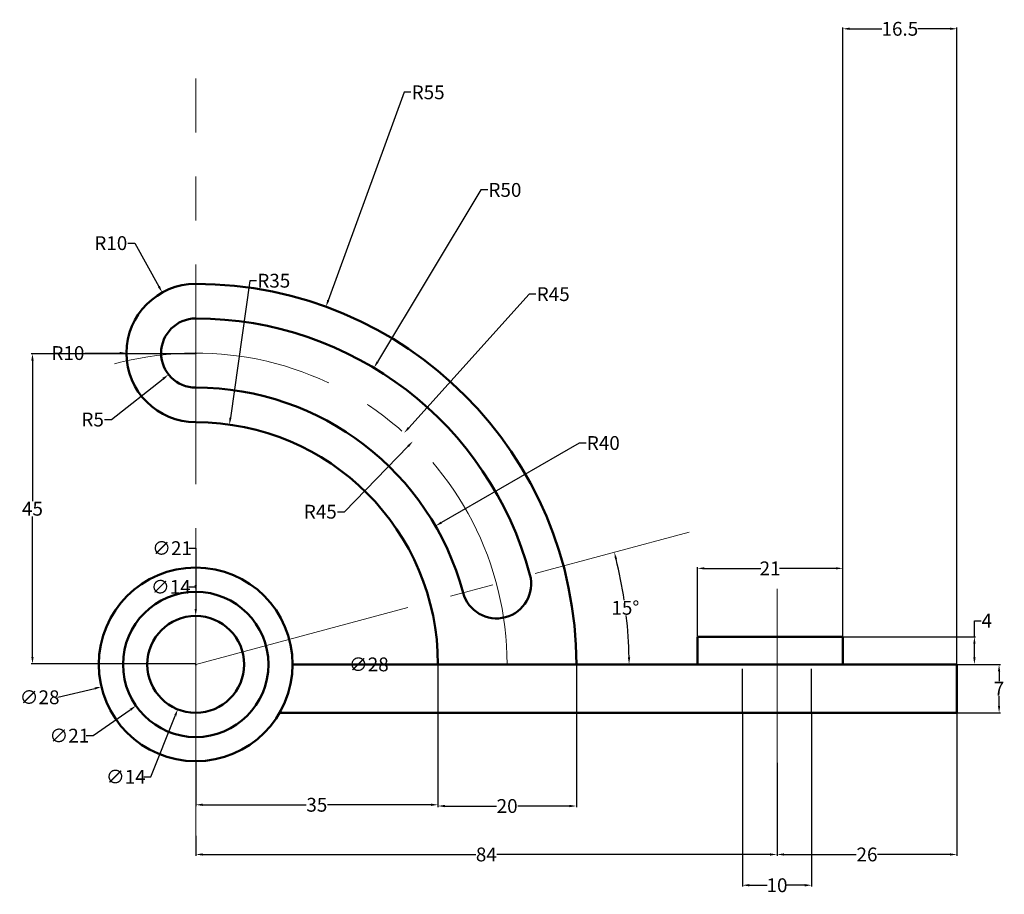
# Model space of a CAD drawing. Units: inches. Extents: x 69 to 212, y 27 to 154.
import ezdxf

# ---------------------------------------------------------------- set-up
doc = ezdxf.new("R2010")
doc.units = ezdxf.units.IN
doc.header["$MEASUREMENT"] = 0
doc.linetypes.add('CENTER', pattern=[50.8, 31.75, -6.35, 6.35, -6.35])
doc.linetypes.add('HIDDEN', pattern=[9.525, 6.35, -3.175])
for name, color, linetype, lineweight in [('M-CNTR', 4, 'CENTER', 18), ('M-DIMS', 2, 'Continuous', 25), ('M-HIDN', 3, 'HIDDEN', 25), ('M-OUTL', 7, 'Continuous', 50)]:
    doc.layers.add(name, color=color, linetype=linetype, lineweight=lineweight)
doc.styles.get("Standard").update_dxf_attribs({"font": 'arial.ttf'})
doc.dimstyles.get("Standard").update_dxf_attribs({"dimtxt": 2, "dimasz": 1, "dimexe": 0.18, "dimexo": 0.0625, "dimgap": 0.09, "dimtad": 0, "dimtih": 1, "dimtoh": 1, "dimdec": 0, "dimzin": 0, "dimdsep": 46, "dimtxsty": 'Standard', "dimcen": 0.09, "dimclrd": 1, "dimclre": 1, "dimadec": 0, "dimazin": 0, "dimtfac": 1, "dimtdec": 0, "dimtofl": 0, "dimtmove": 0, "dimatfit": 3, "dimfxl": 1, "dimtolj": 1, "dimtzin": 0, "dimarcsym": 0})

# ---------------------------------------------------------------- blocks, each defined once
blk = doc.blocks.new('*D1')
at = {"layer": 'Defpoints', "color": 0, "transparency": 16777216}
for p in [(108.33, 63.95), (81.09, 57.47)]:
    blk.add_point(p, dxfattribs=at)
at = {"layer": 'M-DIMS', "color": 0, "lineweight": -2, "transparency": 16777216}
for p, q in [((94.62, 60.71), (94.8, 60.71)), ((94.71, 60.62), (94.71, 60.8)), ((74.77, 55.96), (80.12, 57.24))]:
    blk.add_line(p, q, dxfattribs=at)
at = {"layer": 'M-DIMS', "color": 0, "transparency": 16777216}
blk.add_solid([(80.08, 57.4), (80.16, 57.08), (81.09, 57.47)], dxfattribs=at)
at = {"layer": 'M-DIMS', "color": 0, "transparency": 16777216, "insert": (72.15, 55.96), "char_height": 2, "attachment_point": 5}
blk.add_mtext('\\A1;∅28', dxfattribs=at)
blk = doc.blocks.new('*D2')
at = {"layer": 'Defpoints', "color": 0, "transparency": 16777216}
for p in [(103.34, 66.7), (86.08, 54.73)]:
    blk.add_point(p, dxfattribs=at)
at = {"layer": 'M-DIMS', "color": 0, "lineweight": -2, "transparency": 16777216}
for p, q in [((94.62, 60.71), (94.8, 60.71)), ((94.71, 60.62), (94.71, 60.8)), ((79.87, 50.41), (85.26, 54.16)), ((78.87, 50.41), (79.87, 50.41))]:
    blk.add_line(p, q, dxfattribs=at)
at = {"layer": 'M-DIMS', "color": 0, "transparency": 16777216}
blk.add_solid([(85.17, 54.29), (85.36, 54.02), (86.08, 54.73)], dxfattribs=at)
at = {"layer": 'M-DIMS', "color": 0, "transparency": 16777216, "insert": (76.45, 50.41), "char_height": 2, "attachment_point": 5}
blk.add_mtext('\\A1;∅21', dxfattribs=at)
blk = doc.blocks.new('*D3')
at = {"layer": 'Defpoints', "color": 0, "transparency": 16777216}
for p in [(97.31, 67.21), (92.11, 54.21)]:
    blk.add_point(p, dxfattribs=at)
at = {"layer": 'M-DIMS', "color": 0, "lineweight": -2, "transparency": 16777216}
for p, q in [((94.62, 60.71), (94.8, 60.71)), ((94.71, 60.62), (94.71, 60.8)), ((88.21, 44.47), (91.74, 53.28)), ((87.21, 44.47), (88.21, 44.47))]:
    blk.add_line(p, q, dxfattribs=at)
at = {"layer": 'M-DIMS', "color": 0, "transparency": 16777216}
blk.add_solid([(91.59, 53.35), (91.9, 53.22), (92.11, 54.21)], dxfattribs=at)
at = {"layer": 'M-DIMS', "color": 0, "transparency": 16777216, "insert": (84.61, 44.47), "char_height": 2, "attachment_point": 5}
blk.add_mtext('\\A1;∅14', dxfattribs=at)
blk = doc.blocks.new('*D4')
at = {"layer": 'Defpoints', "color": 0, "transparency": 16777216}
for p in [(129.71, 60.71), (94.71, 46.71), (94.71, 40.42)]:
    blk.add_point(p, dxfattribs=at)
at = {"layer": 'M-DIMS', "color": 0, "lineweight": -2, "transparency": 16777216}
for p, q in [((129.71, 60.65), (129.71, 40.24)), ((94.71, 46.65), (94.71, 40.24)), ((95.71, 40.42), (110.68, 40.42)), ((128.71, 40.42), (113.74, 40.42))]:
    blk.add_line(p, q, dxfattribs=at)
at = {"layer": 'M-DIMS', "color": 0, "transparency": 16777216}
for points in [[(95.71, 40.59), (95.71, 40.25), (94.71, 40.42)], [(128.71, 40.59), (128.71, 40.25), (129.71, 40.42)]]:
    blk.add_solid(points, dxfattribs=at)
at = {"layer": 'M-DIMS', "color": 0, "transparency": 16777216, "insert": (112.21, 40.42), "char_height": 2, "attachment_point": 5}
blk.add_mtext('\\A1;35', dxfattribs=at)
blk = doc.blocks.new('*D5')
at = {"layer": 'Defpoints', "color": 0, "transparency": 16777216}
for p in [(129.71, 60.71), (149.71, 60.71), (129.71, 40.24)]:
    blk.add_point(p, dxfattribs=at)
at = {"layer": 'M-DIMS', "color": 0, "lineweight": -2, "transparency": 16777216}
for p, q in [((129.71, 60.65), (129.71, 40.06)), ((149.71, 60.65), (149.71, 40.06)), ((130.71, 40.24), (138.18, 40.24)), ((148.71, 40.24), (141.25, 40.24))]:
    blk.add_line(p, q, dxfattribs=at)
at = {"layer": 'M-DIMS', "color": 0, "transparency": 16777216}
for points in [[(130.71, 40.41), (130.71, 40.07), (129.71, 40.24)], [(148.71, 40.41), (148.71, 40.07), (149.71, 40.24)]]:
    blk.add_solid(points, dxfattribs=at)
at = {"layer": 'M-DIMS', "color": 0, "transparency": 16777216, "insert": (139.71, 40.24), "char_height": 2, "attachment_point": 5}
blk.add_mtext('\\A1;20', dxfattribs=at)
blk = doc.blocks.new('*D6')
at = {"layer": 'Defpoints', "color": 0, "transparency": 16777216}
for p in [(178.71, 46.52), (94.71, 35.97), (178.71, 33.24)]:
    blk.add_point(p, dxfattribs=at)
at = {"layer": 'M-DIMS', "color": 0, "lineweight": -2, "transparency": 16777216}
for p, q in [((178.71, 46.46), (178.71, 33.06)), ((94.71, 35.91), (94.71, 33.06)), ((95.71, 33.24), (135.19, 33.24)), ((177.71, 33.24), (138.23, 33.24))]:
    blk.add_line(p, q, dxfattribs=at)
at = {"layer": 'M-DIMS', "color": 0, "transparency": 16777216}
for points in [[(95.71, 33.4), (95.71, 33.07), (94.71, 33.24)], [(177.71, 33.4), (177.71, 33.07), (178.71, 33.24)]]:
    blk.add_solid(points, dxfattribs=at)
at = {"layer": 'M-DIMS', "color": 0, "transparency": 16777216, "insert": (136.71, 33.24), "char_height": 2, "attachment_point": 5}
blk.add_mtext('\\A1;84', dxfattribs=at)
blk = doc.blocks.new('*D7')
at = {"layer": 'Defpoints', "color": 0, "transparency": 16777216}
for p in [(204.71, 53.71), (178.71, 46.52), (204.71, 33.24)]:
    blk.add_point(p, dxfattribs=at)
at = {"layer": 'M-DIMS', "color": 0, "lineweight": -2, "transparency": 16777216}
for p, q in [((204.71, 53.65), (204.71, 33.06)), ((178.71, 46.46), (178.71, 33.06)), ((179.71, 33.24), (190.17, 33.24)), ((203.71, 33.24), (193.25, 33.24))]:
    blk.add_line(p, q, dxfattribs=at)
at = {"layer": 'M-DIMS', "color": 0, "transparency": 16777216}
for points in [[(179.71, 33.4), (179.71, 33.07), (178.71, 33.24)], [(203.71, 33.4), (203.71, 33.07), (204.71, 33.24)]]:
    blk.add_solid(points, dxfattribs=at)
at = {"layer": 'M-DIMS', "color": 0, "transparency": 16777216, "insert": (191.71, 33.24), "char_height": 2, "attachment_point": 5}
blk.add_mtext('\\A1;26', dxfattribs=at)
blk = doc.blocks.new('*D8')
at = {"layer": 'Defpoints', "color": 0, "transparency": 16777216}
for p in [(204.71, 60.71), (204.71, 53.71), (210.8, 53.71)]:
    blk.add_point(p, dxfattribs=at)
at = {"layer": 'M-DIMS', "color": 0, "lineweight": -2, "transparency": 16777216}
for p, q in [((204.77, 60.71), (210.98, 60.71)), ((210.8, 59.71), (210.8, 58.3)), ((210.8, 54.71), (210.8, 56.12)), ((204.77, 53.71), (210.98, 53.71))]:
    blk.add_line(p, q, dxfattribs=at)
at = {"layer": 'M-DIMS', "color": 0, "transparency": 16777216}
for points in [[(210.63, 59.71), (210.96, 59.71), (210.8, 60.71)], [(210.63, 54.71), (210.96, 54.71), (210.8, 53.71)]]:
    blk.add_solid(points, dxfattribs=at)
at = {"layer": 'M-DIMS', "color": 0, "transparency": 16777216, "insert": (210.8, 57.21), "char_height": 2, "attachment_point": 5}
blk.add_mtext('\\A1;7', dxfattribs=at)
blk = doc.blocks.new('*D9')
at = {"layer": 'Defpoints', "color": 0, "transparency": 16777216}
for p in [(188.21, 64.71), (188.21, 60.71), (207.23, 60.71)]:
    blk.add_point(p, dxfattribs=at)
at = {"layer": 'M-DIMS', "color": 0, "lineweight": -2, "transparency": 16777216}
for p, q in [((207.23, 64.71), (207.23, 67.02)), ((207.23, 67.02), (208.23, 67.02)), ((188.27, 64.71), (207.41, 64.71)), ((207.23, 61.71), (207.23, 63.71)), ((188.27, 60.71), (207.41, 60.71))]:
    blk.add_line(p, q, dxfattribs=at)
at = {"layer": 'M-DIMS', "color": 0, "transparency": 16777216}
for points in [[(207.07, 63.71), (207.4, 63.71), (207.23, 64.71)], [(207.07, 61.71), (207.4, 61.71), (207.23, 60.71)]]:
    blk.add_solid(points, dxfattribs=at)
at = {"layer": 'M-DIMS', "color": 0, "transparency": 16777216, "insert": (209.01, 67.02), "char_height": 2, "attachment_point": 5}
blk.add_mtext('\\A1;4', dxfattribs=at)
blk = doc.blocks.new('*D10')
at = {"layer": 'Defpoints', "color": 0, "transparency": 16777216}
for p in [(188.21, 74.59), (167.21, 64.71), (188.21, 64.71)]:
    blk.add_point(p, dxfattribs=at)
at = {"layer": 'M-DIMS', "color": 0, "lineweight": -2, "transparency": 16777216}
for p, q in [((167.21, 64.77), (167.21, 74.77)), ((168.21, 74.59), (176.37, 74.59)), ((187.21, 74.59), (179.06, 74.59)), ((188.21, 64.77), (188.21, 74.77))]:
    blk.add_line(p, q, dxfattribs=at)
at = {"layer": 'M-DIMS', "color": 0, "transparency": 16777216}
for points in [[(168.21, 74.76), (168.21, 74.43), (167.21, 74.59)], [(187.21, 74.76), (187.21, 74.43), (188.21, 74.59)]]:
    blk.add_solid(points, dxfattribs=at)
at = {"layer": 'M-DIMS', "color": 0, "transparency": 16777216, "insert": (177.71, 74.59), "char_height": 2, "attachment_point": 5}
blk.add_mtext('\\A1;21', dxfattribs=at)
blk = doc.blocks.new('*D11')
at = {"layer": 'Defpoints', "color": 0, "transparency": 16777216}
for p in [(166.01, 79.82), (157.1, 66.17), (94.71, 60.71), (108.71, 60.71), (178.71, 60.71)]:
    blk.add_point(p, dxfattribs=at)
at = {"layer": 'M-DIMS', "color": 0, "lineweight": -2, "transparency": 16777216}
for start, end in [(8.5267, 14.085), (0.915, 6.4757)]:
    blk.add_arc((94.71, 60.71), 62.62, start, end, dxfattribs=at)
at = {"layer": 'M-DIMS', "color": 0, "transparency": 16777216}
for points in [[(155.29, 75.91), (155.61, 75.99), (155.2, 76.92)], [(157.49, 61.71), (157.16, 61.71), (157.33, 60.71)]]:
    blk.add_solid(points, dxfattribs=at)
at = {"layer": 'M-DIMS', "color": 0, "transparency": 16777216, "insert": (156.8, 68.89), "char_height": 2, "attachment_point": 5}
blk.add_mtext('\\A1;15°', dxfattribs=at)
blk = doc.blocks.new('*D12')
at = {"layer": 'Defpoints', "color": 0, "transparency": 16777216}
for p in [(126.1, 92.96), (94.71, 60.71)]:
    blk.add_point(p, dxfattribs=at)
at = {"layer": 'M-DIMS', "color": 0, "lineweight": -2, "transparency": 16777216}
for p, q in [((116.19, 82.78), (125.4, 92.24)), ((115.19, 82.78), (116.19, 82.78))]:
    blk.add_line(p, q, dxfattribs=at)
at = {"layer": 'M-DIMS', "color": 0, "transparency": 16777216}
blk.add_solid([(125.28, 92.36), (125.52, 92.12), (126.1, 92.96)], dxfattribs=at)
at = {"layer": 'M-DIMS', "color": 0, "transparency": 16777216, "insert": (112.71, 82.78), "char_height": 2, "attachment_point": 5}
blk.add_mtext('\\A1;R45', dxfattribs=at)
blk = doc.blocks.new('*D13')
at = {"layer": 'Defpoints', "color": 0, "transparency": 16777216}
for p in [(94.71, 105.71), (90.79, 102.61)]:
    blk.add_point(p, dxfattribs=at)
at = {"layer": 'M-DIMS', "color": 0, "lineweight": -2, "transparency": 16777216}
for p, q in [((94.62, 105.71), (94.8, 105.71)), ((94.71, 105.62), (94.71, 105.8)), ((82.53, 96.1), (90, 101.99)), ((81.53, 96.1), (82.53, 96.1))]:
    blk.add_line(p, q, dxfattribs=at)
at = {"layer": 'M-DIMS', "color": 0, "transparency": 16777216}
blk.add_solid([(89.9, 102.13), (90.11, 101.86), (90.79, 102.61)], dxfattribs=at)
at = {"layer": 'M-DIMS', "color": 0, "transparency": 16777216, "insert": (79.82, 96.1), "char_height": 2, "attachment_point": 5}
blk.add_mtext('\\A1;R5', dxfattribs=at)
blk = doc.blocks.new('*D14')
at = {"layer": 'Defpoints', "color": 0, "transparency": 16777216}
for p in [(89.87, 114.46), (94.71, 105.71)]:
    blk.add_point(p, dxfattribs=at)
at = {"layer": 'M-DIMS', "color": 0, "lineweight": -2, "transparency": 16777216}
for p, q in [((84.91, 121.6), (85.91, 121.6)), ((85.91, 121.6), (89.38, 115.34)), ((94.62, 105.71), (94.8, 105.71)), ((94.71, 105.62), (94.71, 105.8))]:
    blk.add_line(p, q, dxfattribs=at)
at = {"layer": 'M-DIMS', "color": 0, "transparency": 16777216}
blk.add_solid([(89.53, 115.42), (89.24, 115.25), (89.87, 114.46)], dxfattribs=at)
at = {"layer": 'M-DIMS', "color": 0, "transparency": 16777216, "insert": (82.44, 121.6), "char_height": 2, "attachment_point": 5}
blk.add_mtext('\\A1;R10', dxfattribs=at)
blk = doc.blocks.new('*D15')
at = {"layer": 'Defpoints', "color": 0, "transparency": 16777216}
for p in [(94.71, 105.62), (71.12, 60.8), (94.71, 60.8)]:
    blk.add_point(p, dxfattribs=at)
at = {"layer": 'M-DIMS', "color": 0, "lineweight": -2, "transparency": 16777216}
for p, q in [((94.65, 105.62), (70.94, 105.62)), ((71.12, 104.62), (71.12, 84.32)), ((71.12, 61.8), (71.12, 82.1)), ((94.65, 60.8), (70.94, 60.8))]:
    blk.add_line(p, q, dxfattribs=at)
at = {"layer": 'M-DIMS', "color": 0, "transparency": 16777216}
for points in [[(70.95, 104.62), (71.29, 104.62), (71.12, 105.62)], [(70.95, 61.8), (71.29, 61.8), (71.12, 60.8)]]:
    blk.add_solid(points, dxfattribs=at)
at = {"layer": 'M-DIMS', "color": 0, "transparency": 16777216, "insert": (71.12, 83.21), "char_height": 2, "attachment_point": 5}
blk.add_mtext('\\A1;45', dxfattribs=at)
blk = doc.blocks.new('*D16')
at = {"layer": 'Defpoints', "color": 0, "transparency": 16777216}
for p in [(204.71, 152.58), (188.21, 64.71), (204.71, 60.71)]:
    blk.add_point(p, dxfattribs=at)
at = {"layer": 'M-DIMS', "color": 1, "lineweight": -2, "transparency": 16777216}
for p, q in [((188.21, 64.77), (188.21, 152.76)), ((189.21, 152.58), (193.86, 152.58)), ((203.71, 152.58), (199.06, 152.58)), ((204.71, 60.77), (204.71, 152.76))]:
    blk.add_line(p, q, dxfattribs=at)
at = {"layer": 'M-DIMS', "color": 1, "transparency": 16777216}
for points in [[(189.21, 152.75), (189.21, 152.42), (188.21, 152.58)], [(203.71, 152.75), (203.71, 152.42), (204.71, 152.58)]]:
    blk.add_solid(points, dxfattribs=at)
at = {"layer": 'M-DIMS', "color": 0, "transparency": 16777216, "insert": (196.46, 152.58), "char_height": 2, "attachment_point": 5}
blk.add_mtext('\\A1;16.5', dxfattribs=at)
blk = doc.blocks.new('*D17')
at = {"layer": 'Defpoints', "color": 0, "transparency": 16777216}
for p in [(173.71, 53.71), (183.71, 53.71), (183.71, 28.79)]:
    blk.add_point(p, dxfattribs=at)
at = {"layer": 'M-DIMS', "color": 1, "lineweight": -2, "transparency": 16777216}
for p, q in [((173.71, 53.65), (173.71, 28.61)), ((183.71, 53.65), (183.71, 28.61)), ((174.71, 28.79), (177.29, 28.79)), ((182.71, 28.79), (180.14, 28.79))]:
    blk.add_line(p, q, dxfattribs=at)
at = {"layer": 'M-DIMS', "color": 1, "transparency": 16777216}
for points in [[(174.71, 28.96), (174.71, 28.62), (173.71, 28.79)], [(182.71, 28.96), (182.71, 28.62), (183.71, 28.79)]]:
    blk.add_solid(points, dxfattribs=at)
at = {"layer": 'M-DIMS', "color": 0, "transparency": 16777216, "insert": (178.71, 28.79), "char_height": 2, "attachment_point": 5}
blk.add_mtext('\\A1;10', dxfattribs=at)
blk = doc.blocks.new('*D18')
at = {"layer": 'Defpoints', "color": 0, "transparency": 16777216}
for p in [(113.52, 112.4), (94.71, 60.71)]:
    blk.add_point(p, dxfattribs=at)
at = {"layer": 'M-DIMS', "color": 1, "lineweight": -2, "transparency": 16777216}
for p, q in [((124.81, 143.4), (113.87, 113.33)), ((125.81, 143.4), (124.81, 143.4)), ((94.62, 60.71), (94.8, 60.71)), ((94.71, 60.62), (94.71, 60.8))]:
    blk.add_line(p, q, dxfattribs=at)
at = {"layer": 'M-DIMS', "color": 1, "transparency": 16777216}
blk.add_solid([(113.71, 113.39), (114.02, 113.28), (113.52, 112.4)], dxfattribs=at)
at = {"layer": 'M-DIMS', "color": 0, "transparency": 16777216, "insert": (128.3, 143.4), "char_height": 2, "attachment_point": 5}
blk.add_mtext('\\A1;R55', dxfattribs=at)
blk = doc.blocks.new('*D19')
at = {"layer": 'Defpoints', "color": 0, "transparency": 16777216}
for p in [(120.46, 103.57), (94.71, 60.71)]:
    blk.add_point(p, dxfattribs=at)
at = {"layer": 'M-DIMS', "color": 1, "lineweight": -2, "transparency": 16777216}
for p, q in [((135.92, 129.29), (120.98, 104.43)), ((136.92, 129.29), (135.92, 129.29)), ((94.62, 60.71), (94.8, 60.71)), ((94.71, 60.62), (94.71, 60.8))]:
    blk.add_line(p, q, dxfattribs=at)
at = {"layer": 'M-DIMS', "color": 1, "transparency": 16777216}
blk.add_solid([(120.84, 104.51), (121.12, 104.34), (120.46, 103.57)], dxfattribs=at)
at = {"layer": 'M-DIMS', "color": 0, "transparency": 16777216, "insert": (139.39, 129.29), "char_height": 2, "attachment_point": 5}
blk.add_mtext('\\A1;R50', dxfattribs=at)
blk = doc.blocks.new('*D20')
at = {"layer": 'Defpoints', "color": 0, "transparency": 16777216}
for p in [(124.82, 94.16), (94.71, 60.71)]:
    blk.add_point(p, dxfattribs=at)
at = {"layer": 'M-DIMS', "color": 1, "lineweight": -2, "transparency": 16777216}
for p, q in [((142.88, 114.23), (125.49, 94.9)), ((143.88, 114.23), (142.88, 114.23)), ((94.62, 60.71), (94.8, 60.71)), ((94.71, 60.62), (94.71, 60.8))]:
    blk.add_line(p, q, dxfattribs=at)
at = {"layer": 'M-DIMS', "color": 1, "transparency": 16777216}
blk.add_solid([(125.36, 95.01), (125.61, 94.79), (124.82, 94.16)], dxfattribs=at)
at = {"layer": 'M-DIMS', "color": 0, "transparency": 16777216, "insert": (146.37, 114.23), "char_height": 2, "attachment_point": 5}
blk.add_mtext('\\A1;R45', dxfattribs=at)
blk = doc.blocks.new('*D21')
at = {"layer": 'Defpoints', "color": 0, "transparency": 16777216}
for p in [(129.35, 80.71), (94.71, 60.71)]:
    blk.add_point(p, dxfattribs=at)
at = {"layer": 'M-DIMS', "color": 1, "lineweight": -2, "transparency": 16777216}
for p, q in [((150.14, 92.71), (130.22, 81.21)), ((151.14, 92.71), (150.14, 92.71)), ((94.62, 60.71), (94.8, 60.71)), ((94.71, 60.62), (94.71, 60.8))]:
    blk.add_line(p, q, dxfattribs=at)
at = {"layer": 'M-DIMS', "color": 1, "transparency": 16777216}
blk.add_solid([(130.14, 81.36), (130.3, 81.07), (129.35, 80.71)], dxfattribs=at)
at = {"layer": 'M-DIMS', "color": 0, "transparency": 16777216, "insert": (153.61, 92.71), "char_height": 2, "attachment_point": 5}
blk.add_mtext('\\A1;R40', dxfattribs=at)
blk = doc.blocks.new('*D22')
at = {"layer": 'Defpoints', "color": 0, "transparency": 16777216}
for p in [(99.58, 95.37), (94.71, 60.71)]:
    blk.add_point(p, dxfattribs=at)
at = {"layer": 'M-DIMS', "color": 1, "lineweight": -2, "transparency": 16777216}
for p, q in [((102.51, 116.17), (99.72, 96.36)), ((103.51, 116.17), (102.51, 116.17)), ((94.62, 60.71), (94.8, 60.71)), ((94.71, 60.62), (94.71, 60.8))]:
    blk.add_line(p, q, dxfattribs=at)
at = {"layer": 'M-DIMS', "color": 1, "transparency": 16777216}
blk.add_solid([(99.56, 96.38), (99.89, 96.34), (99.58, 95.37)], dxfattribs=at)
at = {"layer": 'M-DIMS', "color": 0, "transparency": 16777216, "insert": (105.99, 116.17), "char_height": 2, "attachment_point": 5}
blk.add_mtext('\\A1;R35', dxfattribs=at)
blk = doc.blocks.new('*D23')
at = {"layer": 'Defpoints', "color": 0, "transparency": 16777216}
for p in [(80.71, 60.71), (108.71, 60.71)]:
    blk.add_point(p, dxfattribs=at)
at = {"layer": 'M-DIMS', "color": 1, "lineweight": -2, "transparency": 16777216}
for p, q in [((94.62, 60.71), (94.8, 60.71)), ((94.71, 60.62), (94.71, 60.8)), ((117.11, 60.71), (109.71, 60.71))]:
    blk.add_line(p, q, dxfattribs=at)
at = {"layer": 'M-DIMS', "color": 1, "transparency": 16777216}
blk.add_solid([(109.71, 60.88), (109.71, 60.55), (108.71, 60.71)], dxfattribs=at)
at = {"layer": 'M-DIMS', "color": 0, "transparency": 16777216, "insert": (119.72, 60.71), "char_height": 2, "attachment_point": 5}
blk.add_mtext('\\A1;∅28', dxfattribs=at)
blk = doc.blocks.new('*D24')
at = {"layer": 'Defpoints', "color": 0, "transparency": 16777216}
for p in [(94.71, 71.21), (94.71, 50.21)]:
    blk.add_point(p, dxfattribs=at)
at = {"layer": 'M-DIMS', "color": 1, "lineweight": -2, "transparency": 16777216}
for p, q in [((93.71, 77.51), (94.71, 77.51)), ((94.71, 77.51), (94.71, 72.21)), ((94.62, 60.71), (94.8, 60.71)), ((94.71, 60.62), (94.71, 60.8))]:
    blk.add_line(p, q, dxfattribs=at)
at = {"layer": 'M-DIMS', "color": 1, "transparency": 16777216}
blk.add_solid([(94.88, 72.21), (94.55, 72.21), (94.71, 71.21)], dxfattribs=at)
at = {"layer": 'M-DIMS', "color": 0, "transparency": 16777216, "insert": (91.29, 77.51), "char_height": 2, "attachment_point": 5}
blk.add_mtext('\\A1;∅21', dxfattribs=at)
blk = doc.blocks.new('*D25')
at = {"layer": 'Defpoints', "color": 0, "transparency": 16777216}
for p in [(94.71, 67.71), (94.71, 53.71)]:
    blk.add_point(p, dxfattribs=at)
at = {"layer": 'M-DIMS', "color": 1, "lineweight": -2, "transparency": 16777216}
for p, q in [((93.71, 71.91), (94.71, 71.91)), ((94.71, 71.91), (94.71, 68.71)), ((94.62, 60.71), (94.8, 60.71)), ((94.71, 60.62), (94.71, 60.8))]:
    blk.add_line(p, q, dxfattribs=at)
at = {"layer": 'M-DIMS', "color": 1, "transparency": 16777216}
blk.add_solid([(94.88, 68.71), (94.55, 68.71), (94.71, 67.71)], dxfattribs=at)
at = {"layer": 'M-DIMS', "color": 0, "transparency": 16777216, "insert": (91.11, 71.91), "char_height": 2, "attachment_point": 5}
blk.add_mtext('\\A1;∅14', dxfattribs=at)
blk = doc.blocks.new('*D26')
at = {"layer": 'Defpoints', "color": 0, "transparency": 16777216}
for p in [(84.71, 105.71), (94.71, 105.71)]:
    blk.add_point(p, dxfattribs=at)
at = {"layer": 'M-DIMS', "color": 1, "lineweight": -2, "transparency": 16777216}
for p, q in [((78.71, 105.71), (83.71, 105.71)), ((94.62, 105.71), (94.8, 105.71)), ((94.71, 105.62), (94.71, 105.8))]:
    blk.add_line(p, q, dxfattribs=at)
at = {"layer": 'M-DIMS', "color": 1, "transparency": 16777216}
blk.add_solid([(83.71, 105.88), (83.71, 105.55), (84.71, 105.71)], dxfattribs=at)
at = {"layer": 'M-DIMS', "color": 0, "transparency": 16777216, "insert": (76.24, 105.71), "char_height": 2, "attachment_point": 5}
blk.add_mtext('\\A1;R10', dxfattribs=at)

msp = doc.modelspace()

# ---------------------------------------------------------------- linework, layer by layer
at = {"layer": 'M-CNTR'}
for p, q in [((94.71, 35.97), (94.71, 145.4)), ((94.71, 60.71), (166.01, 79.82)), ((178.71, 71.64), (178.71, 46.52))]:
    msp.add_line(p, q, dxfattribs=at)
msp.add_arc((94.71, 60.71), 45, 0, 109.1941, dxfattribs=at)
at = {"layer": 'M-HIDN'}
for p, q in [((173.71, 53.71), (173.71, 60.71)), ((183.71, 53.71), (183.71, 60.71))]:
    msp.add_line(p, q, dxfattribs=at)
at = {"layer": 'M-OUTL'}
for p, q in [((167.21, 60.71), (167.21, 64.71)), ((167.21, 64.71), (188.21, 64.71)), ((188.21, 64.71), (188.21, 60.71)), ((108.71, 60.71), (178.71, 60.71)), ((178.71, 60.71), (204.71, 60.71)), ((204.71, 60.71), (204.71, 53.71)), ((178.71, 53.71), (106.84, 53.71)), ((178.71, 53.71), (173.71, 53.71)), ((204.71, 53.71), (178.71, 53.71)), ((178.71, 53.71), (183.71, 53.71))]:
    msp.add_line(p, q, dxfattribs=at)
for radius in [14, 10.5, 7]:
    msp.add_circle((94.71, 60.71), radius, dxfattribs=at)
for centre, radius, start, end in [((94.71, 105.71), 10, 90, 270), ((94.71, 60.71), 55, 0, 90), ((94.71, 105.71), 5, 90, 270), ((94.71, 60.71), 50, 15, 90), ((94.71, 60.71), 40, 15, 90), ((94.71, 60.71), 35, 0, 90), ((138.18, 72.36), 5, 195, 15)]:
    msp.add_arc(centre, radius, start, end, dxfattribs=at)

# ---------------------------------------------------------------- dimensions: what is measured, and where the dimension line sits
at = {"layer": 'M-DIMS'}
for base, p1, p2, override, picture, middle in [((204.71, 152.58), (188.21, 64.71), (204.71, 60.71), {"dimdec": 1, "dimlfac": 1, "dimrnd": 0, "dimzin": 0, "dimdsep": 46, "dimlunit": 2}, '*D16', (196.46, 152.58)), ((188.21, 74.59), (167.21, 64.71), (188.21, 64.71), {"dimclrd": 0, "dimclre": 0, "dimclrt": 0}, '*D10', (177.71, 74.59)), ((94.71, 40.42), (129.71, 60.71), (94.71, 46.71), {"dimclrd": 0, "dimclre": 0, "dimclrt": 0}, '*D4', (112.21, 40.42)), ((129.71, 40.24), (149.71, 60.71), (129.71, 60.71), {"dimclrd": 0, "dimclre": 0, "dimclrt": 0}, '*D5', (139.71, 40.24)), ((183.71, 28.79), (173.71, 53.71), (183.71, 53.71), {"dimdec": 0, "dimlfac": 1, "dimrnd": 0, "dimzin": 0, "dimdsep": 46, "dimlunit": 2}, '*D17', (178.71, 28.79)), ((204.71, 33.24), (178.71, 46.52), (204.71, 53.71), {"dimclrd": 0, "dimclre": 0, "dimclrt": 0}, '*D7', (191.71, 33.24)), ((178.71, 33.24), (94.71, 35.97), (178.71, 46.52), {"dimclrd": 0, "dimclre": 0, "dimclrt": 0}, '*D6', (136.71, 33.24))]:
    dim = msp.add_linear_dim(base=base, p1=p1, p2=p2, dimstyle='Standard', override=override, dxfattribs=at)
    dim.commit()
    dim.dimension.update_dxf_attribs({"geometry": picture, "text_midpoint": middle})
for center, mpoint, override, picture, middle in [((94.71, 60.71), (113.52, 112.4), {"dimdec": 0, "dimlfac": 1, "dimrnd": 0, "dimzin": 0, "dimdsep": 46, "dimlunit": 2}, '*D18', (128.3, 143.4)), ((94.71, 60.71), (120.46, 103.57), {"dimdec": 0, "dimlfac": 1, "dimrnd": 0, "dimzin": 0, "dimdsep": 46, "dimlunit": 2}, '*D19', (139.39, 129.29)), ((94.71, 105.71), (89.87, 114.46), {"dimclrd": 0, "dimclre": 0, "dimclrt": 0}, '*D14', (82.44, 121.6)), ((94.71, 60.71), (99.58, 95.37), {"dimdec": 0, "dimlfac": 1, "dimrnd": 0, "dimzin": 0, "dimdsep": 46, "dimlunit": 2}, '*D22', (105.99, 116.17)), ((94.71, 60.71), (124.82, 94.16), {"dimdec": 0, "dimlfac": 1, "dimrnd": 0, "dimzin": 0, "dimdsep": 46, "dimlunit": 2}, '*D20', (146.37, 114.23)), ((94.71, 105.71), (84.71, 105.71), {"dimdec": 0, "dimlfac": 1, "dimrnd": 0, "dimzin": 0, "dimdsep": 46, "dimlunit": 2}, '*D26', (78.71, 105.71)), ((94.71, 105.71), (90.79, 102.61), {"dimclrd": 0, "dimclre": 0, "dimclrt": 0}, '*D13', (79.82, 96.1)), ((94.71, 60.71), (129.35, 80.71), {"dimdec": 0, "dimlfac": 1, "dimrnd": 0, "dimzin": 0, "dimdsep": 46, "dimlunit": 2}, '*D21', (153.61, 92.71)), ((94.71, 60.71), (126.1, 92.96), {"dimclrd": 0, "dimclre": 0, "dimclrt": 0}, '*D12', (112.71, 82.78))]:
    dim = msp.add_radius_dim(center=center, mpoint=mpoint, dimstyle='Standard', override=override, dxfattribs=at)
    dim.commit()
    dim.dimension.update_dxf_attribs({"geometry": picture, "text_midpoint": middle, "dimtype": 164})
for base, p1, p2, picture, middle in [((71.12, 60.8), (94.71, 105.62), (94.71, 60.8), '*D15', (71.12, 83.21)), ((210.8, 53.71), (204.71, 60.71), (204.71, 53.71), '*D8', (210.8, 57.21))]:
    dim = msp.add_linear_dim(base=base, p1=p1, p2=p2, angle=90, dimstyle='Standard', override={"dimclrd": 0, "dimclre": 0, "dimclrt": 0}, dxfattribs=at)
    dim.commit()
    dim.dimension.update_dxf_attribs({"geometry": picture, "text_midpoint": middle})
dim = msp.add_angular_dim_2l(base=(157.1, 66.17), line1=((108.71, 60.71), (178.71, 60.71)), line2=((94.71, 60.71), (166.01, 79.82)), dimstyle='Standard', override={"dimclrd": 0, "dimclre": 0, "dimclrt": 0}, dxfattribs=at)
dim.commit()
dim.dimension.update_dxf_attribs({"geometry": '*D11', "text_midpoint": (156.8, 68.89)})
for p1, p2, override, picture, middle in [((94.71, 50.21), (94.71, 71.21), {"dimdec": 0, "dimlfac": 1, "dimrnd": 0, "dimzin": 0, "dimdsep": 46, "dimlunit": 2}, '*D24', (91.29, 77.51)), ((94.71, 53.71), (94.71, 67.71), {"dimdec": 0, "dimlfac": 1, "dimrnd": 0, "dimzin": 0, "dimdsep": 46, "dimlunit": 2}, '*D25', (91.11, 71.91)), ((97.31, 67.21), (92.11, 54.21), {"dimclrd": 0, "dimclre": 0, "dimclrt": 0}, '*D3', (84.61, 44.47)), ((103.34, 66.7), (86.08, 54.73), {"dimclrd": 0, "dimclre": 0, "dimclrt": 0}, '*D2', (76.45, 50.41)), ((108.33, 63.95), (81.09, 57.47), {"dimclrd": 0, "dimclre": 0, "dimclrt": 0}, '*D1', (74.77, 55.96)), ((80.71, 60.71), (108.71, 60.71), {"dimdec": 0, "dimlfac": 1, "dimrnd": 0, "dimzin": 0, "dimdsep": 46, "dimlunit": 2}, '*D23', (117.11, 60.71))]:
    dim = msp.add_diameter_dim_2p(p1=p1, p2=p2, dimstyle='Standard', override=override, dxfattribs=at)
    dim.commit()
    dim.dimension.update_dxf_attribs({"geometry": picture, "text_midpoint": middle, "dimtype": 163})
dim = msp.add_linear_dim(base=(207.23, 60.71), p1=(188.21, 64.71), p2=(188.21, 60.71), angle=90, dimstyle='Standard', override={"dimclrd": 0, "dimclre": 0, "dimclrt": 0}, dxfattribs=at)
dim.commit()
dim.dimension.update_dxf_attribs({"geometry": '*D9', "text_midpoint": (209.01, 67.02), "dimtype": 160})

doc.saveas('drawing.dxf')
